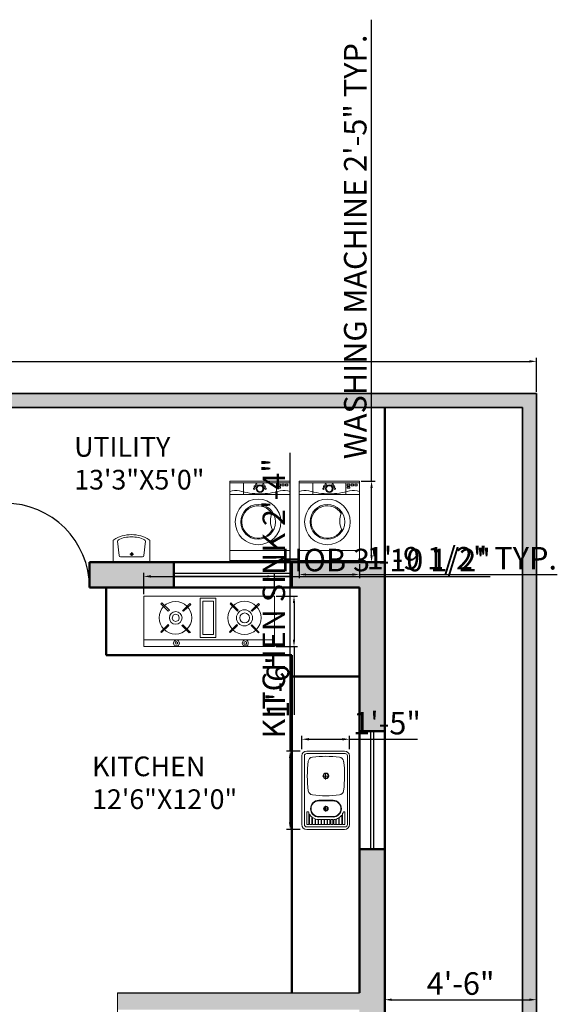
# Model space of a CAD drawing. Units: inches. Extents: x 3008 to 4088, y 1255 to 2137.
# Tile 20 of 30: x 3336 to 3527, y 1787 to 2137. Entities that reach past the tile are written whole.
import ezdxf

# ---------------------------------------------------------------- set-up
doc = ezdxf.new("R2010")
doc.units = ezdxf.units.IN
doc.linetypes.add('DASHED', pattern=[19.05, 12.7, -6.35])
for name, color, linetype, lineweight in [('A-ANNO-DIMS', 2, 'Continuous', 18), ('A-AREA-IDEN', 7, 'Continuous', 18), ('A-DOOR', 4, 'Continuous', 25), ('A-EQPM', 9, 'Continuous', 18), ('A-FLOR-FIXT', 8, 'Continuous', 18), ('A-FLOR-STRS', 3, 'Continuous', 25), ('A-FLOR-STRS-OVHD', 3, 'DASHED', 18), ('A-GLAZ', 4, 'Continuous', 25), ('A-WALL', 7, 'Continuous', 50), ('A-WALL-PATT', 8, 'Continuous', 13), ('C-PROP', 1, 'Continuous', 35), ('C-PROP-PATT', 9, 'Continuous', 13)]:
    doc.layers.add(name, color=color, linetype=linetype, lineweight=lineweight)
doc.styles.get("Standard").update_dxf_attribs({"font": 'arial.ttf'})
doc.dimstyles.new('ISO-25', dxfattribs={"dimtxt": 8, "dimasz": 2.5, "dimexe": 1.25, "dimexo": 0.625, "dimtad": 1, "dimdec": 1, "dimlunit": 3, "dimtxsty": 'Standard', "dimcen": 2.5, "dimadec": 0, "dimazin": 0, "dimtfac": 1, "dimtdec": 1, "dimtmove": 0, "dimatfit": 3, "dimfxl": 1, "dimarcsym": 0})

# ---------------------------------------------------------------- blocks, each defined once
blk = doc.blocks.new('*D1')
at = {"layer": 'A-ANNO-DIMS', "color": 0, "lineweight": -2, "transparency": 16777216}
for p, q in [((3039.67, 2004.59), (3039.67, 2016.66)), ((3519.67, 2004.59), (3519.67, 2016.66)), ((3042.17, 2015.41), (3517.17, 2015.41))]:
    blk.add_line(p, q, dxfattribs=at)
at = {"layer": 'A-ANNO-DIMS', "color": 0, "transparency": 16777216}
for points in [[(3042.17, 2015.82), (3042.17, 2014.99), (3039.67, 2015.41)], [(3517.17, 2015.82), (3517.17, 2014.99), (3519.67, 2015.41)]]:
    blk.add_solid(points, dxfattribs=at)
at = {"layer": 'Defpoints', "color": 0, "transparency": 16777216}
for p in [(3519.67, 2015.41), (3039.67, 2003.97), (3519.67, 2003.97)]:
    blk.add_point(p, dxfattribs=at)
at = {"layer": 'A-ANNO-DIMS', "color": 0, "transparency": 16777216, "insert": (3279.67, 2020.12), "char_height": 8, "attachment_point": 5}
blk.add_mtext("40'", dxfattribs=at)
blk = doc.blocks.new('*D4')
at = {"layer": 'A-ANNO-DIMS', "color": 0, "lineweight": -2, "transparency": 16777216}
for p, q in [((3468.17, 1788.5), (3517.17, 1788.5)), ((3465.67, 1787.88), (3465.67, 1787.25)), ((3519.67, 1787.88), (3519.67, 1787.25))]:
    blk.add_line(p, q, dxfattribs=at)
at = {"layer": 'A-ANNO-DIMS', "color": 0, "transparency": 16777216}
for points in [[(3468.17, 1788.92), (3468.17, 1788.09), (3465.67, 1788.5)], [(3517.17, 1788.92), (3517.17, 1788.09), (3519.67, 1788.5)]]:
    blk.add_solid(points, dxfattribs=at)
at = {"layer": 'Defpoints', "color": 0, "transparency": 16777216}
for p in [(3465.67, 1788.5), (3519.67, 1788.5), (3519.67, 1788.5)]:
    blk.add_point(p, dxfattribs=at)
at = {"layer": 'A-ANNO-DIMS', "color": 0, "transparency": 16777216, "insert": (3492.67, 1793.21), "char_height": 8, "attachment_point": 5}
blk.add_mtext('4\'-6"', dxfattribs=at)
blk = doc.blocks.new('D2')
for p, q in [((1722.5, 1505.46), (1722.5, 1475.46)), ((1723.5, 1505.46), (1723.5, 1475.46)), ((1722.5, 1475.46), (1723.5, 1475.46))]:
    blk.add_line(p, q)
blk.add_arc((1722.5, 1475.46), 30, 0, 90)
blk = doc.blocks.new('sink 1')
for points in [[(-7.34, 1.48), (-7.34, 22.73)], [(-6.56, 1.48), (-6.56, 22.73)], [(5.86, 24.22), (-5.86, 24.22)], [(6.01, 23.43), (-5.86, 23.43)], [(6.72, 1.48), (6.72, 22.73)], [(7.34, 1.48), (7.34, 22.73)], [(1.09, 16.48), (-0.94, 16.48)], [(0, 15.39), (0, 17.42)], [(-2.09, 8.99), (2.28, 8.99)], [(-2.09, 8.84), (2.28, 8.84)], [(0.78, 6.33), (-0.78, 6.33)], [(0, 5.55), (0, 7.26)], [(-5.78, 5.39), (-5.78, 5.39)], [(-5.31, 5.39), (-5.31, 5.39)], [(-5.16, 4.92), (-5.16, 4.92)], [(-5, 1.48), (-5, 4.69)], [(-5, 1.48), (-4.22, 1.48), (-4.22, 3.83)], [(-4.84, 4.45), (-4.84, 4.45)], [(-4.22, 3.83), (-4.22, 3.83)], [(-4.06, 1.48), (-4.06, 3.69)], [(-4.06, 1.48), (-3.28, 1.48), (-3.28, 3.27)], [(-3.91, 3.52), (-3.91, 3.52)], [(-3.28, 3.2), (-3.28, 3.2)], [(-3.12, 3.2), (-3.12, 3.2)], [(-2.34, 3.05), (-2.34, 3.05)], [(-2.19, 3.05), (-2.19, 3.05)], [(-2.09, 3.99), (2.28, 3.99)], [(-2.09, 3.84), (2.28, 3.84)], [(-1.41, 3.05), (-1.41, 3.05)], [(-1.25, 3.05), (-1.25, 3.05)], [(-0.47, 1.48), (-1.25, 1.48), (-1.25, 3.05), (-0.47, 3.05)], [(-0.62, 3.05), (-0.62, 3.05)], [(-0.47, 1.48), (-0.47, 3.05)], [(-0.31, 3.05), (-0.31, 3.05)], [(0.47, 1.48), (-0.31, 1.48), (-0.31, 3.05), (0.47, 3.05)], [(0.31, 3.05), (0.31, 3.05)], [(0.47, 1.48), (0.47, 3.05)], [(0.62, 3.05), (0.62, 3.05)], [(1.25, 3.05), (1.25, 3.05)], [(1.56, 3.05), (1.56, 3.05)], [(2.19, 3.05), (2.19, 3.05)], [(2.5, 3.05), (2.5, 3.05)], [(3.12, 3.2), (3.12, 3.2)], [(3.28, 1.48), (4.06, 1.48), (4.06, 3.57)], [(3.28, 1.48), (3.28, 3.2)], [(3.44, 3.2), (3.44, 3.2)], [(4.06, 3.52), (4.06, 3.52)], [(4.22, 1.48), (4.22, 3.67)], [(4.37, 3.83), (4.37, 3.83)], [(5, 4.45), (5, 4.45)], [(5.16, 4.92), (5.16, 4.92)], [(5.94, 5.39), (5.94, 5.39)], [(6.01, 0.78), (-5.86, 0.78)], [(5.86, 0), (-5.86, 0)], [(-5.78, 1.48), (-5.78, 1.48)], [(-5.16, 1.48), (-5.16, 1.48)], [(-4.84, 1.48), (-4.84, 1.48)], [(-4.22, 1.48), (-4.22, 1.48)], [(-3.91, 1.48), (-3.91, 1.48)], [(-3.28, 1.48), (-3.28, 1.48)], [(-3.12, 1.48), (-3.12, 1.48)], [(-2.34, 1.48), (-2.34, 1.48)], [(-2.19, 1.48), (-2.19, 1.48)], [(-1.41, 1.48), (-1.41, 1.48)], [(-1.25, 1.48), (-1.25, 1.48)], [(-0.62, 1.48), (-0.62, 1.48)], [(-0.31, 1.48), (-0.31, 1.48)], [(0.31, 1.48), (0.31, 1.48)], [(0.62, 1.48), (0.62, 1.48)], [(1.25, 1.48), (1.25, 1.48)], [(1.56, 1.48), (1.56, 1.48)], [(2.19, 1.48), (2.19, 1.48)], [(2.5, 1.48), (2.5, 1.48)], [(3.12, 1.48), (3.12, 1.48)], [(3.44, 1.48), (3.44, 1.48)], [(4.06, 1.48), (4.06, 1.48)], [(4.37, 1.48), (4.37, 1.48)], [(5, 1.48), (5, 1.48)], [(5.16, 1.48), (5.16, 1.48)], [(5.94, 1.48), (5.94, 1.48)]]:
    blk.add_lwpolyline(points)
for points in [[(-5.16, 4.92), (-5.16, 1.48), (-5.78, 1.48), (-5.78, 5.39), (-5.31, 5.39, -0.068511), (-5.16, 4.92)], [(4.06, 3.57, -0.061679), (3.32, 3.22)], [(4.22, 1.48), (5, 1.48), (5, 4.45, -0.083542), (4.22, 3.67, -0.083542)], [(5.16, 4.92, 0.248301), (5.47, 5.39), (5.94, 5.39), (5.94, 1.48), (5.16, 1.48), (5.16, 4.92)]]:
    blk.add_lwpolyline(points, format="xyb")
for points in [[(-3.12, 3.22), (-3.12, 1.48), (-2.34, 1.48), (-2.34, 3.05, -0.06228)], [(2.5, 3.05), (2.5, 1.48), (3.12, 1.48), (3.12, 3.2, -0.050256)]]:
    blk.add_lwpolyline(points, format="xyb", close=True)
for points in [[(-2.19, 3.05), (-1.41, 3.05), (-1.41, 1.48), (-2.19, 1.48)], [(0.62, 3.05), (1.25, 3.05), (1.25, 1.48), (0.62, 1.48)], [(2.19, 1.48), (2.19, 3.05), (1.56, 3.05), (1.56, 1.48)]]:
    blk.add_lwpolyline(points, close=True)
for centre, radius in [((0.09, 16.57), 0.859), ((0.09, 16.57), 0.703), ((0.09, 6.41), 0.703), ((0.09, 6.41), 0.547)]:
    blk.add_circle(centre, radius)
for centre, radius, start, end in [((-5.86, 22.73), 1.48, 90, 180), ((-5.86, 22.73), 0.703, 90, 180), ((-3.87, 20.82), 1.53, 97.3256, 171.1849), ((0.09, -12.65), 35.23, 83.2159, 96.7841), ((4.06, 20.82), 1.53, 8.8151, 82.6744), ((5.86, 22.73), 1.48, 360, 90), ((6.01, 22.73), 0.703, 0, 90), ((30.19, 16.56), 35.85, 172.7947, 187.4213), ((-30, 16.56), 35.85, 352.5787, 7.2053), ((-3.89, 12.12), 1.48, 187.4212, 263.2159), ((0.09, 45.63), 35.23, 263.2159, 276.7841), ((4.08, 12.12), 1.48, 276.7841, 352.5788), ((-2.1, 6.41), 2.58, 90, 270), ((-2.1, 6.41), 2.42, 90, 270), ((2.28, 6.41), 2.58, 270, 90), ((2.28, 6.41), 2.42, 270, 90), ((-2.15, 6.48), 3.36, 212.1095, 232.0862), ((-2.1, 6.41), 3.36, 234.156, 249.3275), ((2.14, 6.36), 3.36, 289.8633, 290.5971), ((-5.86, 1.48), 1.48, 180, 270), ((-5.86, 1.48), 0.703, 180, 270), ((5.86, 1.48), 1.48, 270, 0), ((6.01, 1.48), 0.703, 270, 360)]:
    blk.add_arc(centre, radius, start, end)
blk = doc.blocks.new('A$C2EBB240D')
for p, q in [((0, 356), (0, 87)), ((480, 376), (20, 376)), ((61, 90), (82, 282)), ((250, 300), (102, 300)), ((250, 300), (398, 300)), ((439, 90), (418, 282)), ((500, 356), (500, 87))]:
    blk.add_line(p, q)
for points in [[(247, 238), (247, 289)], [(275, 266), (219, 266)]]:
    blk.add_lwpolyline(points)
for centre, radius, start, end in [((20, 356), 20, 90, 180), ((102, 280), 20, 90, 173.6428), ((247, 266), 16.7, 90, 270), ((247, 266), 10, 90, 270), ((247, 266), 16.7, 270, 90), ((247, 266), 10, 270, 90), ((398, 280), 20, 6.3572, 90), ((480, 356), 20, 0, 90), ((20, 87), 20, 180, 237.6892), ((250, 450), 450, 237.6892, 270), ((81, 88), 20, 173.6428, 244.9796), ((250, 450), 420, 244.9796, 270), ((250, 450), 450, 270, 302.3108), ((250, 450), 420, 270, 295.0204), ((419, 88), 20, 295.0204, 6.3572), ((480, 87), 20, 302.3108, 0)]:
    blk.add_arc(centre, radius, start, end)
blk = doc.blocks.new('gas 1')
for points in [[(35.93, -1.87), (35.93, 0), (0, 0), (0, -1.87)], [(8.12, -0.94), (8.44, -1.56), (8.91, -1.87), (9.53, -1.56), (9.84, -0.94), (9.53, -0.31), (8.91, -0.16), (8.44, -0.31)], [(8.59, -0.94), (8.75, -1.25), (8.91, -1.41), (9.22, -1.25), (9.37, -0.94), (9.22, -0.78), (8.91, -0.62), (8.75, -0.78)], [(19.84, -13.28), (15.47, -13.28), (15.47, -2.5), (19.84, -2.5)], [(27.03, -0.94), (27.34, -1.56), (27.97, -1.87), (28.59, -1.56), (28.75, -0.94), (28.59, -0.31), (27.97, -0.16), (27.34, -0.31)], [(27.5, -0.94), (27.65, -1.25), (27.97, -1.41), (28.28, -1.25), (28.28, -0.94), (28.28, -0.62), (27.97, -0.62), (27.65, -0.62)], [(4.84, -3.91), (4.69, -4.06), (6.72, -6.09), (6.87, -5.78)], [(12.81, -3.91), (12.5, -3.75), (10.47, -5.78), (10.78, -5.94)], [(19.22, -12.5), (16.25, -12.5), (16.25, -3.28), (19.22, -3.28)], [(23.75, -3.91), (23.59, -4.06), (25.62, -6.09), (25.78, -5.78)], [(31.71, -3.91), (31.56, -3.75), (29.53, -5.78), (29.68, -5.94)], [(7.81, -7.81), (8.12, -8.59), (8.75, -8.91), (9.53, -8.59), (9.69, -7.81), (9.53, -7.19), (8.75, -6.87), (8.12, -7.19)], [(7.03, -10), (6.72, -9.69), (4.69, -11.72), (5, -12.03)], [(12.97, -11.56), (10.94, -9.69), (10.62, -9.84), (12.65, -11.87)], [(23.75, -11.72), (23.9, -12.03), (25.93, -10), (25.78, -9.69)], [(31.87, -11.56), (29.84, -9.69), (29.53, -9.84), (31.56, -11.87)]]:
    blk.add_lwpolyline(points, close=True)
blk.add_lwpolyline([(35.93, -1.87), (35.93, -13.9), (0, -13.9), (0, -1.87)])
for centre, radius in [((8.7, -7.92), 4.48), ((27.7, -7.86), 4.58), ((8.77, -7.89), 1.74), ((27.69, -7.89), 2.22), ((27.76, -7.89), 1.35)]:
    blk.add_circle(centre, radius)
blk = doc.blocks.new('WASHING-MACHINE')
for p, q in [((0.21, -0.03), (0.21, 28.86)), ((0.21, 28.86), (21.67, 28.86)), ((0.21, 28.17), (21.67, 28.17)), ((5.06, 24.02), (5.06, 28.17)), ((16.82, 24.02), (16.82, 28.17)), ((21.67, -0.03), (21.67, 28.86)), ((0.21, 24.02), (21.67, 24.02)), ((0.21, 4.12), (21.67, 4.12)), ((0.21, 0.66), (21.67, 0.66)), ((0.21, -0.03), (21.67, -0.03))]:
    blk.add_line(p, q)
for points in [[(17.38, 27.7), (18.28, 27.7), (18.28, 27.2), (17.38, 27.2)], [(17.38, 26.83), (18.28, 26.83), (18.28, 26.32), (17.38, 26.32)], [(18.7, 27.7), (19.6, 27.7), (19.6, 27.2), (18.7, 27.2)], [(20.02, 27.7), (20.91, 27.7), (20.91, 27.2), (20.02, 27.2)]]:
    blk.add_lwpolyline(points, close=True)
for centre, radius in [((8.89, 26.12), 0.271), ((9.14, 26.91), 0.271), ((9.67, 27.64), 0.271), ((10.94, 26.12), 1.34), ((10.94, 26.12), 1.07), ((12.19, 27.64), 0.271), ((12.67, 26.91), 0.271), ((12.93, 26.12), 0.271), ((10.29, 14.33), 8.1), ((10.29, 14.33), 6.17)]:
    blk.add_circle(centre, radius)
for centre, radius, start, end in [((2.28, 20.66), 4.89, 73.3932, 115.105), ((11.47, 54.22), 29.92, 254.9063, 268.9794), ((10.41, 54.22), 29.92, 271.0206, 285.0937), ((19.59, 20.66), 4.89, 64.895, 106.6068), ((10.29, 14.33), 5.77, 31.8067, 332.1506), ((21.49, 14.71), 6.83, 153.19, 210.7673)]:
    blk.add_arc(centre, radius, start, end)
blk = doc.blocks.new('*D59')
at = {"layer": 'A-ANNO-DIMS', "color": 0, "lineweight": -2, "transparency": 16777216}
for p, q in [((3461, 1972.86), (3461, 2136.84)), ((3457.29, 1972.86), (3462.25, 1972.86)), ((3461, 1946.47), (3461, 1970.36)), ((3457.29, 1943.97), (3462.25, 1943.97))]:
    blk.add_line(p, q, dxfattribs=at)
at = {"layer": 'A-ANNO-DIMS', "color": 0, "transparency": 16777216}
for points in [[(3460.58, 1970.36), (3461.42, 1970.36), (3461, 1972.86)], [(3460.58, 1946.47), (3461.42, 1946.47), (3461, 1943.97)]]:
    blk.add_solid(points, dxfattribs=at)
at = {"layer": 'Defpoints', "color": 0, "transparency": 16777216}
for p in [(3456.67, 1972.86), (3461, 1972.86), (3456.67, 1943.97)]:
    blk.add_point(p, dxfattribs=at)
at = {"layer": 'A-ANNO-DIMS', "color": 0, "transparency": 16777216, "insert": (3456.24, 2056.1), "char_height": 8, "attachment_point": 5, "rotation": 90}
blk.add_mtext('WASHING MACHINE 2\'-5" TYP.', dxfattribs=at)
blk = doc.blocks.new('*D60')
at = {"layer": 'A-ANNO-DIMS', "color": 0, "lineweight": -2, "transparency": 16777216}
for p, q in [((3435.21, 1943.34), (3435.21, 1938.38)), ((3456.67, 1943.34), (3456.67, 1938.38)), ((3437.71, 1939.63), (3454.17, 1939.63)), ((3456.67, 1939.63), (3527.07, 1939.63))]:
    blk.add_line(p, q, dxfattribs=at)
at = {"layer": 'A-ANNO-DIMS', "color": 0, "transparency": 16777216}
for points in [[(3437.71, 1940.05), (3437.71, 1939.22), (3435.21, 1939.63)], [(3454.17, 1940.05), (3454.17, 1939.22), (3456.67, 1939.63)]]:
    blk.add_solid(points, dxfattribs=at)
at = {"layer": 'Defpoints', "color": 0, "transparency": 16777216}
for p in [(3435.21, 1943.97), (3456.67, 1943.97), (3456.67, 1939.63)]:
    blk.add_point(p, dxfattribs=at)
at = {"layer": 'A-ANNO-DIMS', "color": 0, "transparency": 16777216, "insert": (3493.12, 1944.39), "char_height": 8, "attachment_point": 5}
blk.add_mtext('1\'-9 1/2" TYP.', dxfattribs=at)
blk = doc.blocks.new('*D67')
at = {"layer": 'A-ANNO-DIMS', "color": 0, "lineweight": -2, "transparency": 16777216}
for p, q in [((3432.04, 1876.9), (3432.04, 1982.91)), ((3435.59, 1876.9), (3430.79, 1876.9)), ((3432.04, 1851.53), (3432.04, 1874.4)), ((3435.59, 1849.03), (3430.79, 1849.03))]:
    blk.add_line(p, q, dxfattribs=at)
at = {"layer": 'A-ANNO-DIMS', "color": 0, "transparency": 16777216}
for points in [[(3431.62, 1874.4), (3432.45, 1874.4), (3432.04, 1876.9)], [(3431.62, 1851.53), (3432.45, 1851.53), (3432.04, 1849.03)]]:
    blk.add_solid(points, dxfattribs=at)
at = {"layer": 'Defpoints', "color": 0, "transparency": 16777216}
for p in [(3432.04, 1876.9), (3436.22, 1876.9), (3436.22, 1849.03)]:
    blk.add_point(p, dxfattribs=at)
at = {"layer": 'A-ANNO-DIMS', "color": 0, "transparency": 16777216, "insert": (3427.27, 1931.15), "char_height": 8, "attachment_point": 5, "rotation": 90}
blk.add_mtext('KITCHEN SINK 2\'-4"', dxfattribs=at)
blk = doc.blocks.new('*D68')
at = {"layer": 'A-ANNO-DIMS', "color": 0, "lineweight": -2, "transparency": 16777216}
for p, q in [((3436.22, 1877.52), (3436.22, 1882.33)), ((3438.72, 1881.08), (3450.62, 1881.08)), ((3453.12, 1877.52), (3453.12, 1882.33)), ((3453.12, 1881.08), (3477.38, 1881.08))]:
    blk.add_line(p, q, dxfattribs=at)
at = {"layer": 'A-ANNO-DIMS', "color": 0, "transparency": 16777216}
for points in [[(3438.72, 1881.5), (3438.72, 1880.66), (3436.22, 1881.08)], [(3450.62, 1881.5), (3450.62, 1880.66), (3453.12, 1881.08)]]:
    blk.add_solid(points, dxfattribs=at)
at = {"layer": 'Defpoints', "color": 0, "transparency": 16777216}
for p in [(3453.12, 1881.08), (3436.22, 1876.9), (3453.12, 1876.9)]:
    blk.add_point(p, dxfattribs=at)
at = {"layer": 'A-ANNO-DIMS', "color": 0, "transparency": 16777216, "insert": (3466.5, 1885.79), "char_height": 8, "attachment_point": 5}
blk.add_mtext('1\'-5"', dxfattribs=at)
blk = doc.blocks.new('*D69')
at = {"layer": 'A-ANNO-DIMS', "color": 0, "lineweight": -2, "transparency": 16777216}
for p, q in [((3380, 1932.63), (3380, 1940.22)), ((3382.5, 1938.97), (3423.95, 1938.97)), ((3426.45, 1932.63), (3426.45, 1940.22)), ((3426.45, 1938.97), (3503.22, 1938.97))]:
    blk.add_line(p, q, dxfattribs=at)
at = {"layer": 'A-ANNO-DIMS', "color": 0, "transparency": 16777216}
for points in [[(3382.5, 1939.39), (3382.5, 1938.55), (3380, 1938.97)], [(3423.95, 1939.39), (3423.95, 1938.55), (3426.45, 1938.97)]]:
    blk.add_solid(points, dxfattribs=at)
at = {"layer": 'Defpoints', "color": 0, "transparency": 16777216}
for p in [(3426.45, 1938.97), (3380, 1932), (3426.45, 1932)]:
    blk.add_point(p, dxfattribs=at)
at = {"layer": 'A-ANNO-DIMS', "color": 0, "transparency": 16777216, "insert": (3466.08, 1943.74), "char_height": 8, "attachment_point": 5}
blk.add_mtext('HOB 3\'-10 1/2"', dxfattribs=at)
blk = doc.blocks.new('*D70')
at = {"layer": 'A-ANNO-DIMS', "color": 0, "lineweight": -2, "transparency": 16777216}
for p, q in [((3427.08, 1932), (3434.67, 1932)), ((3433.42, 1929.5), (3433.42, 1916.53)), ((3427.08, 1914.03), (3434.67, 1914.03)), ((3433.42, 1914.03), (3433.42, 1889.77))]:
    blk.add_line(p, q, dxfattribs=at)
at = {"layer": 'A-ANNO-DIMS', "color": 0, "transparency": 16777216}
for points in [[(3433, 1929.5), (3433.83, 1929.5), (3433.42, 1932)], [(3433, 1916.53), (3433.83, 1916.53), (3433.42, 1914.03)]]:
    blk.add_solid(points, dxfattribs=at)
at = {"layer": 'Defpoints', "color": 0, "transparency": 16777216}
for p in [(3426.45, 1932), (3426.45, 1914.03), (3433.42, 1914.03)]:
    blk.add_point(p, dxfattribs=at)
at = {"layer": 'A-ANNO-DIMS', "color": 0, "transparency": 16777216, "insert": (3428.71, 1900.65), "char_height": 8, "attachment_point": 5, "rotation": 90}
blk.add_mtext('1\'-6"', dxfattribs=at)

msp = doc.modelspace()

# ---------------------------------------------------------------- hatches: boundary and pattern name
at = {"layer": 'A-WALL-PATT'}
h = msp.add_hatch(color=256, dxfattribs=at)
h.dxf.hatch_style = 1
h.paths.add_polyline_path([(3102.67, 1625.97), (3093.67, 1625.97), (3093.67, 1540.97), (3102.67, 1540.97)])
h.paths.add_polyline_path([(3102.67, 1784.97), (3252.67, 1784.97), (3252.67, 1790.97), (3102.67, 1790.97), (3102.67, 1892.97), (3093.67, 1892.97), (3093.67, 1667.97), (3102.67, 1667.97)])
h.paths.add_polyline_path([(3192.67, 1943.97), (3093.67, 1943.97), (3093.67, 1934.97), (3102.67, 1934.97), (3192.67, 1934.97)])
h.paths.add_polyline_path([(3264.67, 1943.97), (3234.67, 1943.97), (3234.67, 1934.97), (3246.67, 1934.97), (3246.67, 1868.97), (3252.67, 1868.97), (3252.67, 1934.97), (3264.67, 1934.97)])
h.paths.add_polyline_path([(3330.67, 1943.97), (3288.67, 1943.97), (3288.67, 1934.97), (3300.67, 1934.97), (3300.67, 1838.97), (3246.67, 1838.97), (3246.67, 1826.97), (3252.67, 1826.97), (3252.67, 1832.97), (3306.67, 1832.97), (3306.67, 1934.97), (3330.67, 1934.97)])
h.paths.add_polyline_path([(3390.67, 1943.97), (3360.67, 1943.97), (3360.67, 1934.97), (3390.67, 1934.97)])
h.paths.add_polyline_path([(3465.67, 1943.97), (3432.67, 1943.97), (3432.67, 1934.97), (3456.67, 1934.97), (3456.67, 1883.97), (3465.67, 1883.97)])
h.paths.add_polyline_path([(3465.67, 1841.97), (3456.67, 1841.97), (3456.67, 1790.97), (3370.67, 1790.97), (3370.67, 1784.97), (3456.67, 1784.97), (3456.67, 1759.47), (3465.67, 1759.47)])
h.paths.add_polyline_path([(3465.67, 1693.47), (3456.67, 1693.47), (3456.67, 1667.97), (3330.67, 1667.97), (3330.67, 1643.97), (3336.67, 1643.97), (3336.67, 1661.97), (3456.67, 1661.97), (3456.67, 1649.97), (3465.67, 1649.97)])
h.paths.add_polyline_path([(3465.67, 1625.97), (3456.67, 1625.97), (3456.67, 1613.97), (3324.67, 1613.97), (3324.67, 1604.97), (3456.67, 1604.97), (3456.67, 1571.97), (3465.67, 1571.97)])
h.paths.add_polyline_path([(3465.67, 1505.97), (3456.67, 1505.97), (3456.67, 1472.97), (3438.67, 1472.97), (3438.67, 1463.97), (3465.67, 1463.97)])
h.paths.add_polyline_path([(3396.67, 1472.97), (3354.67, 1472.97), (3354.67, 1463.97), (3396.67, 1463.97)])
h.paths.add_polyline_path([(3312.67, 1472.97), (3288.67, 1472.97), (3288.67, 1550.97), (3282.67, 1550.97), (3282.67, 1472.97), (3270.67, 1472.97), (3270.67, 1463.97), (3312.67, 1463.97)])
h.paths.add_polyline_path([(3246.67, 1472.97), (3234.67, 1472.97), (3234.67, 1544.97), (3252.67, 1544.97), (3252.67, 1550.97), (3234.67, 1550.97), (3234.67, 1604.97), (3282.67, 1604.97), (3282.67, 1580.97), (3288.67, 1580.97), (3288.67, 1613.97), (3150.67, 1613.97), (3150.67, 1604.97), (3225.67, 1604.97), (3225.67, 1463.97), (3246.67, 1463.97)])
at = {"layer": 'C-PROP-PATT'}
h = msp.add_hatch(color=256, dxfattribs=at)
h.dxf.hatch_style = 1
h.paths.add_polyline_path([(3519.67, 2003.97), (3039.67, 2003.97), (3039.67, 1343.97), (3051.67, 1343.97), (3051.67, 1348.97), (3044.67, 1348.97), (3044.67, 1998.97), (3514.67, 1998.97), (3514.67, 1348.97), (3219.67, 1348.97), (3219.67, 1343.97), (3519.67, 1343.97)])

# ---------------------------------------------------------------- linework, layer by layer
at = {"layer": 'A-FLOR-STRS'}
msp.add_line((3370.67, 1790.97), (3456.67, 1790.97), dxfattribs=at)
at = {"layer": 'A-FLOR-STRS-OVHD'}
msp.add_line((3370.67, 1790.97), (3370.67, 1748.97), dxfattribs=at)
at = {"layer": 'A-GLAZ'}
for p, q in [((3432.67, 1939.97), (3390.67, 1939.97)), ((3432.67, 1938.97), (3390.67, 1938.97)), ((3460.67, 1883.97), (3460.67, 1841.97)), ((3460.67, 1883.97), (3460.67, 1841.97)), ((3461.67, 1883.97), (3461.67, 1841.97))]:
    msp.add_line(p, q, dxfattribs=at)
at = {"layer": 'A-WALL'}
for p, q in [((3465.67, 1998.97), (3465.67, 1463.97)), ((3360.67, 1943.97), (3360.67, 1934.97)), ((3360.67, 1943.97), (3465.67, 1943.97)), ((3390.67, 1934.97), (3390.67, 1943.97)), ((3432.67, 1934.97), (3432.67, 1943.97)), ((3360.67, 1934.97), (3456.67, 1934.97)), ((3366.67, 1934.97), (3366.67, 1910.97)), ((3456.67, 1934.97), (3456.67, 1790.97)), ((3366.67, 1910.97), (3432.67, 1910.97)), ((3432.67, 1910.97), (3432.67, 1790.97)), ((3432.67, 1903.43), (3456.67, 1903.43)), ((3456.67, 1883.97), (3465.67, 1883.97)), ((3456.67, 1841.97), (3465.67, 1841.97))]:
    msp.add_line(p, q, dxfattribs=at)
at = {"layer": 'C-PROP'}
for p, q in [((3039.67, 2003.97), (3519.67, 2003.97)), ((3519.67, 2003.97), (3519.67, 1343.97)), ((3044.67, 1998.97), (3514.67, 1998.97)), ((3514.67, 1998.97), (3514.67, 1348.97))]:
    msp.add_line(p, q, dxfattribs=at)

# ---------------------------------------------------------------- block references
at = {"layer": 'A-DOOR'}
msp.add_blockref('D2', (1608.17, 459.51), dxfattribs=at)
at = {"layer": 'A-EQPM'}
for p in [(3410.35, 1944), (3435, 1944)]:
    msp.add_blockref('WASHING-MACHINE', p, dxfattribs=at)
at = {"layer": 'A-FLOR-FIXT', "rotation": 180}
for name, p, xscale, yscale, zscale in [('A$C2EBB240D', (3382.18, 1953.82), 0.026211548048557, 0.026211548048557, 0.026211548048557), ('gas 1', (3380, 1914.03), -1.292580420916565, 1.292580420916565, 1.292580420916565)]:
    msp.add_blockref(name, p, dxfattribs=dict(at, xscale=xscale, yscale=yscale, zscale=zscale))
at = {"layer": 'A-FLOR-FIXT', "xscale": 1.150769176553845, "yscale": 1.150769176553845, "zscale": 1.150769176553845}
msp.add_blockref('sink 1', (3444.67, 1849.03), dxfattribs=at)

# ---------------------------------------------------------------- texts
at = {"layer": 'A-AREA-IDEN', "char_height": 7, "attachment_point": 1}
for s, insert in [('{\\fTimes New Roman|b0|i0|c0|p18;UTILITY\\P13\'3"X5\'0"}', (3355.23, 1988.51)), ('{\\fTimes New Roman|b0|i0|c0|p18;KITCHEN\\P12\'6"X12\'0"}', (3361.59, 1874.95))]:
    msp.add_mtext_dynamic_manual_height_columns(s, width=105.6127, gutter_width=12.5, heights=[0], dxfattribs=dict(at, insert=insert))

# ---------------------------------------------------------------- dimensions: what is measured, and where the dimension line sits
at = {"layer": 'A-ANNO-DIMS'}
for base, p1, p2, text, picture, middle in [((3461, 1972.86), (3456.67, 1943.97), (3456.67, 1972.86), 'WASHING MACHINE <> TYP.', '*D59', (3456.24, 2056.1)), ((3432.04, 1876.9), (3436.22, 1849.03), (3436.22, 1876.9), 'KITCHEN SINK <>', '*D67', (3427.27, 1931.15))]:
    dim = msp.add_linear_dim(base=base, p1=p1, p2=p2, angle=90, text=text, dimstyle='ISO-25', override={"dimdec": 1, "dimrnd": 0, "dimzin": 1, "dimlunit": 4, "dimfrac": 2}, dxfattribs=at)
    dim.commit()
    dim.dimension.update_dxf_attribs({"geometry": picture, "text_midpoint": middle})
for base, p1, p2, override, picture, middle in [((3519.67, 2015.41), (3039.67, 2003.97), (3519.67, 2003.97), {"dimclrd": 0, "dimclre": 0, "dimclrt": 0}, '*D1', (3279.67, 2020.12)), ((3453.12, 1881.08), (3436.22, 1876.9), (3453.12, 1876.9), {"dimdec": 1, "dimrnd": 0, "dimzin": 1, "dimlunit": 4, "dimfrac": 2}, '*D68', (3466.5, 1885.79)), ((3519.67, 1788.5), (3465.67, 1788.5), (3519.67, 1788.5), {"dimclrd": 0, "dimclre": 0, "dimclrt": 0}, '*D4', (3492.67, 1793.21))]:
    dim = msp.add_linear_dim(base=base, p1=p1, p2=p2, dimstyle='ISO-25', override=override, dxfattribs=at)
    dim.commit()
    dim.dimension.update_dxf_attribs({"geometry": picture, "text_midpoint": middle})
for base, p1, p2, text, picture, middle in [((3426.4509, 1938.9702), (3380.0044, 1932.0032), (3426.4509, 1932.0032), 'HOB <>', '*D69', (3466.0834, 1943.737)), ((3456.67, 1939.63), (3435.21, 1943.97), (3456.67, 1943.97), '<> TYP.', '*D60', (3493.12, 1944.39))]:
    dim = msp.add_linear_dim(base=base, p1=p1, p2=p2, text=text, dimstyle='ISO-25', override={"dimdec": 1, "dimrnd": 0, "dimzin": 1, "dimlunit": 4, "dimfrac": 2}, dxfattribs=at)
    dim.commit()
    dim.dimension.update_dxf_attribs({"geometry": picture, "text_midpoint": middle})
dim = msp.add_linear_dim(base=(3433.42, 1914.03), p1=(3426.45, 1932), p2=(3426.45, 1914.03), angle=270, dimstyle='ISO-25', override={"dimdec": 1, "dimrnd": 0, "dimzin": 1, "dimlunit": 4, "dimfrac": 2}, dxfattribs=at)
dim.commit()
dim.dimension.update_dxf_attribs({"geometry": '*D70', "text_midpoint": (3428.71, 1900.65)})

doc.saveas('drawing.dxf')
